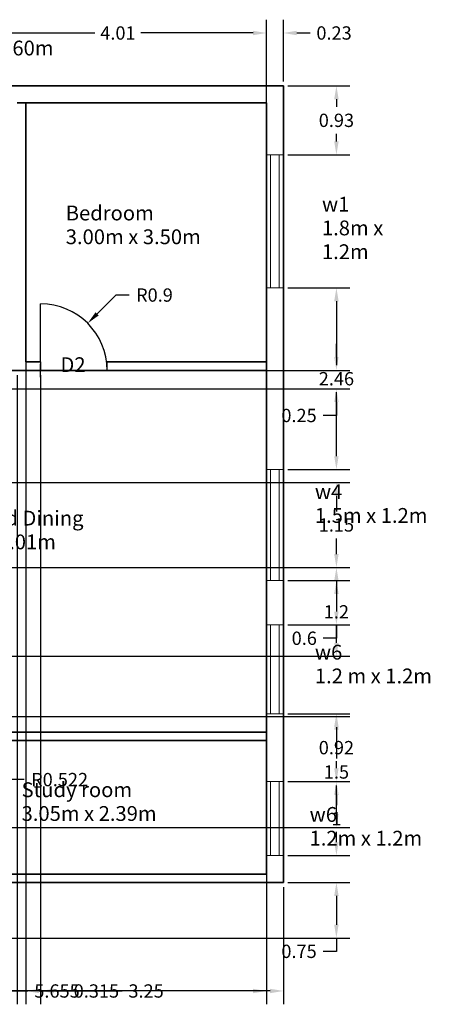
# Model space of a CAD drawing. Units: metres. Extents: x 1585.4 to 1599.4, y 2063.3 to 2076.9.
# Tile 3 of 3: x 1593.9 to 1599.4, y 2063.3 to 2076.6. Entities that reach past the tile are written whole.
import ezdxf

# ---------------------------------------------------------------- set-up
doc = ezdxf.new("R2010")
doc.units = ezdxf.units.M
for name, color, linetype, lineweight in [('A-ANNO-DIMS', 2, 'Continuous', 18), ('A-ANNO-TEXT', 7, 'Continuous', 18), ('A-AREA-IDEN', 7, 'Continuous', 18), ('A-DOOR', 3, 'Continuous', 25), ('A-GLAZ', 4, 'Continuous', 18), ('A-WALL', 7, 'Continuous', 35)]:
    doc.layers.add(name, color=color, linetype=linetype, lineweight=lineweight)
doc.styles.get("Standard").update_dxf_attribs({"font": 'arial.ttf'})
doc.dimstyles.get("Standard").update_dxf_attribs({"dimtxt": 0.18, "dimasz": 0.18, "dimexe": 0.18, "dimexo": 0.0625, "dimgap": 0.09, "dimtad": 0, "dimtih": 1, "dimtoh": 1, "dimdec": 4, "dimzin": 0, "dimdsep": 46, "dimtxsty": 'Standard', "dimcen": 0.09, "dimadec": 0, "dimazin": 0, "dimtfac": 1, "dimtdec": 4, "dimtofl": 0, "dimtmove": 0, "dimatfit": 3, "dimfxl": 1, "dimtolj": 1, "dimtzin": 0, "dimarcsym": 0})

# ---------------------------------------------------------------- blocks, each defined once
blk = doc.blocks.new('WIN-FRAME-1800')
for p, q in [((0, 0), (0, 0.23)), ((0, 0.23), (1.8, 0.23)), ((1.8, 0.23), (1.8, 0))]:
    blk.add_line(p, q)
blk = doc.blocks.new('WIN-FRAME-1500')
for p, q in [((0, 0), (0, 0.23)), ((0, 0.23), (1.5, 0.23)), ((1.5, 0.23), (1.5, 0))]:
    blk.add_line(p, q)
blk = doc.blocks.new('WIN-FRAME-1000')
for p, q in [((0, 0), (0, 1)), ((0, 1), (0.23, 1)), ((0.23, 0), (0, 0))]:
    blk.add_line(p, q)
blk = doc.blocks.new('WIN-FRAME-1200')
for p, q in [((0, 0), (0, 1.2)), ((0, 1.2), (0.23, 1.2)), ((0.23, 0), (0, 0))]:
    blk.add_line(p, q)
blk = doc.blocks.new('*D6')
at = {"layer": 'A-ANNO-DIMS', "color": 0, "lineweight": -2, "transparency": 16777216}
for p, q in [((1586.931, 2064.876), (1586.931, 2063.293)), ((1597.431, 2064.876), (1597.431, 2063.293)), ((1587.111, 2063.473), (1591.865, 2063.473)), ((1597.251, 2063.473), (1592.497, 2063.473))]:
    blk.add_line(p, q, dxfattribs=at)
at = {"layer": 'A-ANNO-DIMS', "color": 0, "transparency": 16777216}
for points in [[(1587.111, 2063.503), (1587.111, 2063.443), (1586.931, 2063.473)], [(1597.251, 2063.503), (1597.251, 2063.443), (1597.431, 2063.473)]]:
    blk.add_solid(points, dxfattribs=at)
at = {"layer": 'Defpoints', "color": 0, "transparency": 16777216}
for p in [(1586.931, 2064.939), (1597.431, 2064.939), (1597.431, 2063.473)]:
    blk.add_point(p, dxfattribs=at)
at = {"layer": 'A-ANNO-DIMS', "color": 0, "transparency": 16777216, "insert": (1592.181, 2063.473), "char_height": 0.18, "attachment_point": 5}
blk.add_mtext('\\A1;10.5', dxfattribs=at)
blk = doc.blocks.new('*D9')
at = {"layer": 'A-ANNO-DIMS', "color": 0, "lineweight": -2, "transparency": 16777216}
for p, q in [((1597.201, 2075.541), (1597.201, 2076.605)), ((1597.431, 2075.771), (1597.431, 2076.605)), ((1597.021, 2076.425), (1596.841, 2076.425)), ((1597.611, 2076.425), (1597.791, 2076.425))]:
    blk.add_line(p, q, dxfattribs=at)
at = {"layer": 'A-ANNO-DIMS', "color": 0, "transparency": 16777216}
for points in [[(1597.021, 2076.455), (1597.021, 2076.395), (1597.201, 2076.425)], [(1597.611, 2076.455), (1597.611, 2076.395), (1597.431, 2076.425)]]:
    blk.add_solid(points, dxfattribs=at)
at = {"layer": 'Defpoints', "color": 0, "transparency": 16777216}
for p in [(1597.431, 2076.425), (1597.431, 2075.709), (1597.201, 2075.479)]:
    blk.add_point(p, dxfattribs=at)
at = {"layer": 'A-ANNO-DIMS', "color": 0, "transparency": 16777216, "insert": (1598.115, 2076.425), "char_height": 0.18, "attachment_point": 5}
blk.add_mtext('\\A1;0.23', dxfattribs=at)
blk = doc.blocks.new('*D10')
at = {"layer": 'A-ANNO-DIMS', "color": 0, "lineweight": -2, "transparency": 16777216}
for p, q in [((1597.493, 2064.939), (1598.327, 2064.939)), ((1598.147, 2064.759), (1598.147, 2064.369)), ((1593.112, 2064.189), (1598.327, 2064.189)), ((1598.147, 2064.189), (1598.147, 2064.009)), ((1598.147, 2064.009), (1597.967, 2064.009))]:
    blk.add_line(p, q, dxfattribs=at)
at = {"layer": 'A-ANNO-DIMS', "color": 0, "transparency": 16777216}
for points in [[(1598.117, 2064.759), (1598.177, 2064.759), (1598.147, 2064.939)], [(1598.117, 2064.369), (1598.177, 2064.369), (1598.147, 2064.189)]]:
    blk.add_solid(points, dxfattribs=at)
at = {"layer": 'Defpoints', "color": 0, "transparency": 16777216}
for p in [(1597.431, 2064.939), (1593.05, 2064.189), (1598.147, 2064.189)]:
    blk.add_point(p, dxfattribs=at)
at = {"layer": 'A-ANNO-DIMS', "color": 0, "transparency": 16777216, "insert": (1597.642, 2064.009), "char_height": 0.18, "attachment_point": 5}
blk.add_mtext('\\A1;0.75', dxfattribs=at)
blk = doc.blocks.new('*D14')
at = {"layer": 'A-ANNO-DIMS', "color": 0, "lineweight": -2, "transparency": 16777216}
for p, q in [((1597.493, 2075.709), (1598.327, 2075.709)), ((1598.147, 2075.529), (1598.147, 2075.426)), ((1598.147, 2074.959), (1598.147, 2075.062)), ((1597.493, 2074.779), (1598.327, 2074.779))]:
    blk.add_line(p, q, dxfattribs=at)
at = {"layer": 'A-ANNO-DIMS', "color": 0, "transparency": 16777216}
for points in [[(1598.117, 2075.529), (1598.177, 2075.529), (1598.147, 2075.709)], [(1598.117, 2074.959), (1598.177, 2074.959), (1598.147, 2074.779)]]:
    blk.add_solid(points, dxfattribs=at)
at = {"layer": 'Defpoints', "color": 0, "transparency": 16777216}
for p in [(1597.431, 2075.709), (1597.431, 2074.779), (1598.147, 2074.779)]:
    blk.add_point(p, dxfattribs=at)
at = {"layer": 'A-ANNO-DIMS', "color": 0, "transparency": 16777216, "insert": (1598.147, 2075.244), "char_height": 0.18, "attachment_point": 5}
blk.add_mtext('\\A1;0.93', dxfattribs=at)
blk = doc.blocks.new('*D15')
at = {"layer": 'A-ANNO-DIMS', "color": 0, "lineweight": -2, "transparency": 16777216}
for p, q in [((1597.493, 2072.979), (1598.327, 2072.979)), ((1598.147, 2072.799), (1598.147, 2071.932)), ((1598.147, 2070.702), (1598.147, 2071.569)), ((1597.493, 2070.522), (1598.327, 2070.522))]:
    blk.add_line(p, q, dxfattribs=at)
at = {"layer": 'A-ANNO-DIMS', "color": 0, "transparency": 16777216}
for points in [[(1598.117, 2072.799), (1598.177, 2072.799), (1598.147, 2072.979)], [(1598.117, 2070.702), (1598.177, 2070.702), (1598.147, 2070.522)]]:
    blk.add_solid(points, dxfattribs=at)
at = {"layer": 'Defpoints', "color": 0, "transparency": 16777216}
for p in [(1597.431, 2072.979), (1597.431, 2070.522), (1598.147, 2070.522)]:
    blk.add_point(p, dxfattribs=at)
at = {"layer": 'A-ANNO-DIMS', "color": 0, "transparency": 16777216, "insert": (1598.147, 2071.751), "char_height": 0.18, "attachment_point": 5}
blk.add_mtext('\\A1;2.46', dxfattribs=at)
blk = doc.blocks.new('*D16')
at = {"layer": 'A-ANNO-DIMS', "color": 0, "lineweight": -2, "transparency": 16777216}
for p, q in [((1597.493, 2069.022), (1598.327, 2069.022)), ((1598.147, 2068.842), (1598.147, 2068.602)), ((1597.493, 2068.422), (1598.327, 2068.422)), ((1598.147, 2068.422), (1598.147, 2068.242)), ((1598.147, 2068.242), (1597.967, 2068.242))]:
    blk.add_line(p, q, dxfattribs=at)
at = {"layer": 'A-ANNO-DIMS', "color": 0, "transparency": 16777216}
for points in [[(1598.117, 2068.842), (1598.177, 2068.842), (1598.147, 2069.022)], [(1598.117, 2068.602), (1598.177, 2068.602), (1598.147, 2068.422)]]:
    blk.add_solid(points, dxfattribs=at)
at = {"layer": 'Defpoints', "color": 0, "transparency": 16777216}
for p in [(1597.431, 2069.022), (1597.431, 2068.422), (1598.147, 2068.422)]:
    blk.add_point(p, dxfattribs=at)
at = {"layer": 'A-ANNO-DIMS', "color": 0, "transparency": 16777216, "insert": (1597.713, 2068.242), "char_height": 0.18, "attachment_point": 5}
blk.add_mtext('\\A1;0.6', dxfattribs=at)
blk = doc.blocks.new('*D17')
at = {"layer": 'A-ANNO-DIMS', "color": 0, "lineweight": -2, "transparency": 16777216}
for p, q in [((1597.493, 2067.222), (1598.327, 2067.222)), ((1598.147, 2067.042), (1598.147, 2066.945)), ((1598.147, 2066.484), (1598.147, 2066.581)), ((1597.493, 2066.304), (1598.327, 2066.304))]:
    blk.add_line(p, q, dxfattribs=at)
at = {"layer": 'A-ANNO-DIMS', "color": 0, "transparency": 16777216}
for points in [[(1598.117, 2067.042), (1598.177, 2067.042), (1598.147, 2067.222)], [(1598.117, 2066.484), (1598.177, 2066.484), (1598.147, 2066.304)]]:
    blk.add_solid(points, dxfattribs=at)
at = {"layer": 'Defpoints', "color": 0, "transparency": 16777216}
for p in [(1597.431, 2067.222), (1597.431, 2066.304), (1598.147, 2066.304)]:
    blk.add_point(p, dxfattribs=at)
at = {"layer": 'A-ANNO-DIMS', "color": 0, "transparency": 16777216, "insert": (1598.147, 2066.763), "char_height": 0.18, "attachment_point": 5}
blk.add_mtext('\\A1;0.92', dxfattribs=at)
blk = doc.blocks.new('*D18')
at = {"layer": 'A-ANNO-DIMS', "color": 0, "lineweight": -2, "transparency": 16777216}
for p, q in [((1597.493, 2066.304), (1598.327, 2066.304)), ((1598.147, 2066.124), (1598.147, 2065.984)), ((1598.147, 2065.484), (1598.147, 2065.623)), ((1597.493, 2065.304), (1598.327, 2065.304))]:
    blk.add_line(p, q, dxfattribs=at)
at = {"layer": 'A-ANNO-DIMS', "color": 0, "transparency": 16777216}
for points in [[(1598.117, 2066.124), (1598.177, 2066.124), (1598.147, 2066.304)], [(1598.117, 2065.484), (1598.177, 2065.484), (1598.147, 2065.304)]]:
    blk.add_solid(points, dxfattribs=at)
at = {"layer": 'Defpoints', "color": 0, "transparency": 16777216}
for p in [(1597.431, 2066.304), (1597.431, 2065.304), (1598.147, 2065.304)]:
    blk.add_point(p, dxfattribs=at)
at = {"layer": 'A-ANNO-DIMS', "color": 0, "transparency": 16777216, "insert": (1598.147, 2065.804), "char_height": 0.18, "attachment_point": 5}
blk.add_mtext('\\A1;1', dxfattribs=at)
blk = doc.blocks.new('*D19')
at = {"layer": 'A-ANNO-DIMS', "color": 0, "lineweight": -2, "transparency": 16777216}
for p, q in [((1587.223, 2070.349), (1598.327, 2070.349)), ((1598.147, 2070.169), (1598.147, 2069.956)), ((1598.147, 2069.379), (1598.147, 2069.592)), ((1587.223, 2069.199), (1598.327, 2069.199))]:
    blk.add_line(p, q, dxfattribs=at)
at = {"layer": 'A-ANNO-DIMS', "color": 0, "transparency": 16777216}
for points in [[(1598.117, 2070.169), (1598.177, 2070.169), (1598.147, 2070.349)], [(1598.117, 2069.379), (1598.177, 2069.379), (1598.147, 2069.199)]]:
    blk.add_solid(points, dxfattribs=at)
at = {"layer": 'Defpoints', "color": 0, "transparency": 16777216}
for p in [(1587.161, 2070.349), (1587.161, 2069.199), (1598.147, 2069.199)]:
    blk.add_point(p, dxfattribs=at)
at = {"layer": 'A-ANNO-DIMS', "color": 0, "transparency": 16777216, "insert": (1598.147, 2069.774), "char_height": 0.18, "attachment_point": 5}
blk.add_mtext('\\A1;1.15', dxfattribs=at)
blk = doc.blocks.new('*D20')
at = {"layer": 'A-ANNO-DIMS', "color": 0, "lineweight": -2, "transparency": 16777216}
for p, q in [((1587.223, 2069.199), (1598.327, 2069.199)), ((1598.147, 2069.019), (1598.147, 2068.779)), ((1598.147, 2068.179), (1598.147, 2068.418)), ((1587.223, 2067.999), (1598.327, 2067.999))]:
    blk.add_line(p, q, dxfattribs=at)
at = {"layer": 'A-ANNO-DIMS', "color": 0, "transparency": 16777216}
for points in [[(1598.117, 2069.019), (1598.177, 2069.019), (1598.147, 2069.199)], [(1598.117, 2068.179), (1598.177, 2068.179), (1598.147, 2067.999)]]:
    blk.add_solid(points, dxfattribs=at)
at = {"layer": 'Defpoints', "color": 0, "transparency": 16777216}
for p in [(1587.161, 2069.199), (1598.147, 2069.199), (1587.161, 2067.999)]:
    blk.add_point(p, dxfattribs=at)
at = {"layer": 'A-ANNO-DIMS', "color": 0, "transparency": 16777216, "insert": (1598.147, 2068.599), "char_height": 0.18, "attachment_point": 5}
blk.add_mtext('\\A1;1.2', dxfattribs=at)
blk = doc.blocks.new('*D21')
at = {"layer": 'A-ANNO-DIMS', "color": 0, "lineweight": -2, "transparency": 16777216}
for p, q in [((1598.147, 2072.044), (1598.147, 2072.224)), ((1587.223, 2071.864), (1598.327, 2071.864)), ((1587.223, 2071.614), (1598.327, 2071.614)), ((1598.147, 2071.434), (1598.147, 2071.254)), ((1598.147, 2071.254), (1597.967, 2071.254))]:
    blk.add_line(p, q, dxfattribs=at)
at = {"layer": 'A-ANNO-DIMS', "color": 0, "transparency": 16777216}
for points in [[(1598.117, 2072.044), (1598.177, 2072.044), (1598.147, 2071.864)], [(1598.117, 2071.434), (1598.177, 2071.434), (1598.147, 2071.614)]]:
    blk.add_solid(points, dxfattribs=at)
at = {"layer": 'Defpoints', "color": 0, "transparency": 16777216}
for p in [(1587.161, 2071.864), (1587.161, 2071.614), (1598.147, 2071.614)]:
    blk.add_point(p, dxfattribs=at)
at = {"layer": 'A-ANNO-DIMS', "color": 0, "transparency": 16777216, "insert": (1597.642, 2071.254), "char_height": 0.18, "attachment_point": 5}
blk.add_mtext('\\A1;0.25', dxfattribs=at)
blk = doc.blocks.new('*D24')
at = {"layer": 'A-ANNO-DIMS', "color": 0, "lineweight": -2, "transparency": 16777216}
for p, q in [((1593.951, 2075.416), (1593.951, 2063.293)), ((1597.201, 2075.416), (1597.201, 2063.293)), ((1594.131, 2063.473), (1595.251, 2063.473)), ((1597.021, 2063.473), (1595.9, 2063.473))]:
    blk.add_line(p, q, dxfattribs=at)
at = {"layer": 'A-ANNO-DIMS', "color": 0, "transparency": 16777216}
for points in [[(1594.131, 2063.503), (1594.131, 2063.443), (1593.951, 2063.473)], [(1597.021, 2063.503), (1597.021, 2063.443), (1597.201, 2063.473)]]:
    blk.add_solid(points, dxfattribs=at)
at = {"layer": 'Defpoints', "color": 0, "transparency": 16777216}
for p in [(1593.951, 2075.479), (1597.201, 2075.479), (1597.201, 2063.473)]:
    blk.add_point(p, dxfattribs=at)
at = {"layer": 'A-ANNO-DIMS', "color": 0, "transparency": 16777216, "insert": (1595.576, 2063.473), "char_height": 0.18, "attachment_point": 5}
blk.add_mtext('\\A1;3.25', dxfattribs=at)
blk = doc.blocks.new('*D25')
at = {"layer": 'A-ANNO-DIMS', "color": 0, "lineweight": -2, "transparency": 16777216}
for p, q in [((1597.138, 2066.857), (1586.035, 2066.857)), ((1586.215, 2066.677), (1586.215, 2066.137)), ((1586.215, 2065.234), (1586.215, 2065.774)), ((1597.138, 2065.054), (1586.035, 2065.054))]:
    blk.add_line(p, q, dxfattribs=at)
at = {"layer": 'A-ANNO-DIMS', "color": 0, "transparency": 16777216}
for points in [[(1586.185, 2066.677), (1586.245, 2066.677), (1586.215, 2066.857)], [(1586.185, 2065.234), (1586.245, 2065.234), (1586.215, 2065.054)]]:
    blk.add_solid(points, dxfattribs=at)
at = {"layer": 'Defpoints', "color": 0, "transparency": 16777216}
for p in [(1586.215, 2066.857), (1597.201, 2066.857), (1597.201, 2065.054)]:
    blk.add_point(p, dxfattribs=at)
at = {"layer": 'A-ANNO-DIMS', "color": 0, "transparency": 16777216, "insert": (1586.215, 2065.956), "char_height": 0.18, "attachment_point": 5}
blk.add_mtext('\\A1;1.80', dxfattribs=at)
blk = doc.blocks.new('*D26')
at = {"layer": 'A-ANNO-DIMS', "color": 0, "lineweight": -2, "transparency": 16777216}
for p, q in [((1593.191, 2065.116), (1593.191, 2076.605)), ((1597.201, 2065.116), (1597.201, 2076.605)), ((1593.371, 2076.425), (1594.886, 2076.425)), ((1597.021, 2076.425), (1595.506, 2076.425))]:
    blk.add_line(p, q, dxfattribs=at)
at = {"layer": 'A-ANNO-DIMS', "color": 0, "transparency": 16777216}
for points in [[(1593.371, 2076.455), (1593.371, 2076.395), (1593.191, 2076.425)], [(1597.021, 2076.455), (1597.021, 2076.395), (1597.201, 2076.425)]]:
    blk.add_solid(points, dxfattribs=at)
at = {"layer": 'Defpoints', "color": 0, "transparency": 16777216}
for p in [(1597.201, 2076.425), (1593.191, 2065.054), (1597.201, 2065.054)]:
    blk.add_point(p, dxfattribs=at)
at = {"layer": 'A-ANNO-DIMS', "color": 0, "transparency": 16777216, "insert": (1595.196, 2076.425), "char_height": 0.18, "attachment_point": 5}
blk.add_mtext('\\A1;4.01', dxfattribs=at)
blk = doc.blocks.new('*D29')
at = {"layer": 'A-ANNO-DIMS', "color": 0, "lineweight": -2, "transparency": 16777216}
for p, q in [((1590.216, 2067.184), (1598.327, 2067.184)), ((1598.147, 2067.004), (1598.147, 2066.616)), ((1598.147, 2065.864), (1598.147, 2066.252)), ((1590.216, 2065.684), (1598.327, 2065.684))]:
    blk.add_line(p, q, dxfattribs=at)
at = {"layer": 'A-ANNO-DIMS', "color": 0, "transparency": 16777216}
for points in [[(1598.117, 2067.004), (1598.177, 2067.004), (1598.147, 2067.184)], [(1598.117, 2065.864), (1598.177, 2065.864), (1598.147, 2065.684)]]:
    blk.add_solid(points, dxfattribs=at)
at = {"layer": 'Defpoints', "color": 0, "transparency": 16777216}
for p in [(1590.153, 2067.184), (1590.153, 2065.684), (1598.147, 2065.684)]:
    blk.add_point(p, dxfattribs=at)
at = {"layer": 'A-ANNO-DIMS', "color": 0, "transparency": 16777216, "insert": (1598.147, 2066.434), "char_height": 0.18, "attachment_point": 5}
blk.add_mtext('\\A1;1.5', dxfattribs=at)
blk = doc.blocks.new('*D31')
at = {"layer": 'A-ANNO-DIMS', "color": 0, "lineweight": -2, "transparency": 16777216}
for p, q in [((1593.836, 2071.801), (1593.836, 2063.293)), ((1594.151, 2071.801), (1594.151, 2063.293)), ((1593.656, 2063.473), (1593.476, 2063.473)), ((1594.331, 2063.473), (1594.511, 2063.473))]:
    blk.add_line(p, q, dxfattribs=at)
at = {"layer": 'A-ANNO-DIMS', "color": 0, "transparency": 16777216}
for points in [[(1593.656, 2063.503), (1593.656, 2063.443), (1593.836, 2063.473)], [(1594.331, 2063.503), (1594.331, 2063.443), (1594.151, 2063.473)]]:
    blk.add_solid(points, dxfattribs=at)
at = {"layer": 'Defpoints', "color": 0, "transparency": 16777216}
for p in [(1593.836, 2071.864), (1594.151, 2071.864), (1594.151, 2063.473)]:
    blk.add_point(p, dxfattribs=at)
at = {"layer": 'A-ANNO-DIMS', "color": 0, "transparency": 16777216, "insert": (1594.905, 2063.473), "char_height": 0.18, "attachment_point": 5}
blk.add_mtext('\\A1;0.315', dxfattribs=at)
blk = doc.blocks.new('*D36')
at = {"layer": 'A-ANNO-DIMS', "color": 0, "lineweight": -2, "transparency": 16777216}
for p, q in [((1597.201, 2070.46), (1597.201, 2063.293)), ((1591.546, 2070.401), (1591.546, 2063.293)), ((1591.726, 2063.473), (1593.979, 2063.473)), ((1597.021, 2063.473), (1594.768, 2063.473))]:
    blk.add_line(p, q, dxfattribs=at)
at = {"layer": 'A-ANNO-DIMS', "color": 0, "transparency": 16777216}
for points in [[(1591.726, 2063.503), (1591.726, 2063.443), (1591.546, 2063.473)], [(1597.021, 2063.503), (1597.021, 2063.443), (1597.201, 2063.473)]]:
    blk.add_solid(points, dxfattribs=at)
at = {"layer": 'Defpoints', "color": 0, "transparency": 16777216}
for p in [(1591.546, 2070.464), (1597.201, 2070.522), (1597.201, 2063.473)]:
    blk.add_point(p, dxfattribs=at)
at = {"layer": 'A-ANNO-DIMS', "color": 0, "transparency": 16777216, "insert": (1594.373, 2063.473), "char_height": 0.18, "attachment_point": 5}
blk.add_mtext('\\A1;5.655', dxfattribs=at)
blk = doc.blocks.new('*D37')
at = {"layer": 'A-ANNO-DIMS', "color": 0, "lineweight": -2, "transparency": 16777216}
for p, q in [((1597.138, 2071.864), (1586.035, 2071.864)), ((1586.215, 2071.684), (1586.215, 2069.6)), ((1586.215, 2067.152), (1586.215, 2069.236)), ((1597.138, 2066.972), (1586.035, 2066.972))]:
    blk.add_line(p, q, dxfattribs=at)
at = {"layer": 'A-ANNO-DIMS', "color": 0, "transparency": 16777216}
for points in [[(1586.185, 2071.684), (1586.245, 2071.684), (1586.215, 2071.864)], [(1586.185, 2067.152), (1586.245, 2067.152), (1586.215, 2066.972)]]:
    blk.add_solid(points, dxfattribs=at)
at = {"layer": 'Defpoints', "color": 0, "transparency": 16777216}
for p in [(1586.215, 2071.864), (1597.201, 2071.864), (1597.201, 2066.972)]:
    blk.add_point(p, dxfattribs=at)
at = {"layer": 'A-ANNO-DIMS', "color": 0, "transparency": 16777216, "insert": (1586.215, 2069.418), "char_height": 0.18, "attachment_point": 5}
blk.add_mtext('\\A1;4.892', dxfattribs=at)
blk = doc.blocks.new('*D39')
at = {"layer": 'A-ANNO-DIMS', "color": 0, "lineweight": -2, "transparency": 16777216}
for p, q in [((1595.169, 2072.882), (1594.915, 2072.628)), ((1595.349, 2072.882), (1595.169, 2072.882)), ((1594.151, 2071.774), (1594.151, 2071.954)), ((1594.061, 2071.864), (1594.241, 2071.864))]:
    blk.add_line(p, q, dxfattribs=at)
at = {"layer": 'A-ANNO-DIMS', "color": 0, "transparency": 16777216}
blk.add_solid([(1594.893, 2072.649), (1594.936, 2072.606), (1594.787, 2072.5)], dxfattribs=at)
at = {"layer": 'Defpoints', "color": 0, "transparency": 16777216}
for p in [(1594.787, 2072.5), (1594.151, 2071.864)]:
    blk.add_point(p, dxfattribs=at)
at = {"layer": 'A-ANNO-DIMS', "color": 0, "transparency": 16777216, "insert": (1595.689, 2072.882), "char_height": 0.18, "attachment_point": 5}
blk.add_mtext('\\A1;R0.9', dxfattribs=at)
blk = doc.blocks.new('*D43')
at = {"layer": 'A-ANNO-DIMS', "color": 0, "lineweight": -2, "transparency": 16777216}
for p, q in [((1592.951, 2066.857), (1593.131, 2066.857)), ((1593.041, 2066.767), (1593.041, 2066.947)), ((1593.749, 2066.331), (1593.604, 2066.439)), ((1593.929, 2066.331), (1593.749, 2066.331))]:
    blk.add_line(p, q, dxfattribs=at)
at = {"layer": 'A-ANNO-DIMS', "color": 0, "transparency": 16777216}
blk.add_solid([(1593.622, 2066.463), (1593.587, 2066.415), (1593.46, 2066.546)], dxfattribs=at)
at = {"layer": 'Defpoints', "color": 0, "transparency": 16777216}
for p in [(1593.041, 2066.857), (1593.46, 2066.546)]:
    blk.add_point(p, dxfattribs=at)
at = {"layer": 'A-ANNO-DIMS', "color": 0, "transparency": 16777216, "insert": (1594.408, 2066.331), "char_height": 0.18, "attachment_point": 5}
blk.add_mtext('\\A1;R0.522', dxfattribs=at)

msp = doc.modelspace()

# ---------------------------------------------------------------- linework, layer by layer
at = {"layer": 'A-DOOR'}
for p, q in [((1594.1508, 2071.9788), (1594.1508, 2072.7638)), ((1594.1508, 2071.9788), (1594.1508, 2071.8638)), ((1595.0508, 2071.8638), (1595.0508, 2071.9788))]:
    msp.add_line(p, q, dxfattribs=at)
msp.add_arc((1594.1508, 2071.8638), 0.9, 0, 90, dxfattribs=at)
at = {"layer": 'A-GLAZ'}
for p, q in [((1597.2008, 2072.9788), (1597.2008, 2074.7788)), ((1597.2558, 2072.9788), (1597.2558, 2074.7788)), ((1597.3758, 2072.9788), (1597.3758, 2074.7788)), ((1597.2558, 2069.0223), (1597.2558, 2070.5223)), ((1597.3758, 2069.0223), (1597.3758, 2070.5223)), ((1597.2558, 2067.2223), (1597.2558, 2068.4223)), ((1597.3758, 2067.2223), (1597.3758, 2068.4223)), ((1597.2008, 2065.3038), (1597.2008, 2066.3038)), ((1597.2558, 2065.3038), (1597.2558, 2066.3038)), ((1597.3758, 2065.3038), (1597.3758, 2066.3038))]:
    msp.add_line(p, q, dxfattribs=at)
at = {"layer": 'A-WALL'}
for p, q in [((1597.4308, 2075.7088), (1597.2008, 2075.7088)), ((1593.9508, 2075.4788), (1593.8358, 2075.4788)), ((1597.2008, 2075.4788), (1593.9508, 2075.4788)), ((1593.9508, 2075.4788), (1593.9508, 2071.9788)), ((1597.2008, 2071.9788), (1597.2008, 2075.4788)), ((1597.2008, 2071.9788), (1597.2008, 2072.9788)), ((1593.9508, 2071.9788), (1594.1508, 2071.9788)), ((1593.9508, 2071.9788), (1594.1508, 2071.9788)), ((1595.0508, 2071.9788), (1597.2008, 2071.9788)), ((1597.2008, 2071.9788), (1597.2008, 2071.9788)), ((1593.8358, 2071.8638), (1594.1508, 2071.8638)), ((1595.0508, 2071.8638), (1597.2008, 2071.8638)), ((1597.2008, 2071.8638), (1597.2008, 2066.9723)), ((1597.2008, 2068.4223), (1597.2008, 2069.0223)), ((1597.2008, 2068.4223), (1597.2008, 2068.4223)), ((1597.2008, 2066.9723), (1597.2008, 2067.3288)), ((1597.2008, 2066.9723), (1597.2008, 2067.2223)), ((1597.2008, 2066.9723), (1593.0408, 2066.9723)), ((1593.1908, 2066.8573), (1597.2008, 2066.8573)), ((1597.2008, 2065.0538), (1597.2008, 2066.8573)), ((1597.2008, 2066.8573), (1597.2008, 2065.0538)), ((1597.2008, 2065.0538), (1597.2008, 2065.3038)), ((1597.2008, 2065.0538), (1593.1908, 2065.0538)), ((1593.0458, 2064.9388), (1597.2008, 2064.9388)), ((1597.2008, 2064.9388), (1597.4308, 2064.9388))]:
    msp.add_line(p, q, dxfattribs=at)
msp.add_lwpolyline([(1597.4308, 2064.9388), (1597.4308, 2075.7088), (1586.9308, 2075.7088), (1586.9308, 2064.9388)], dxfattribs=at)

# ---------------------------------------------------------------- block references
at = {"layer": 'A-GLAZ'}
for name, p, rotation in [('WIN-FRAME-1800', (1597.2008, 2074.7788), 269.9999999999952), ('WIN-FRAME-1500', (1597.2008, 2070.5223), 270), ('WIN-FRAME-1200', (1597.4308, 2068.4223), 180), ('WIN-FRAME-1000', (1597.4308, 2066.3038), 180)]:
    msp.add_blockref(name, p, dxfattribs=dict(at, rotation=rotation))

# ---------------------------------------------------------------- texts
at = {"layer": 'A-ANNO-TEXT'}
for s, p in [('0.9m x 0.60m', (1592.6536, 2076.1214)), ('w1', (1597.9517, 2074.0105)), ('1.8m x', (1597.9517, 2073.6892)), ('1.2m', (1597.9517, 2073.3679)), ('D2', (1594.4197, 2071.8405)), ('w4', (1597.8563, 2070.1236)), ('1.5m x 1.2m', (1597.8563, 2069.8023)), ('w6', (1597.8563, 2067.9537)), ('1.2 m x 1.2m', (1597.8563, 2067.6324)), ('w6', (1597.7847, 2065.7599)), ('1.2m x 1.2m', (1597.7847, 2065.4386))]:
    msp.add_text(s, height=0.2, dxfattribs=at).set_placement(p)
at = {"layer": 'A-AREA-IDEN'}
for s, p in [('Bedroom', (1594.4913, 2073.8912)), ('3.00m x 3.50m', (1594.4913, 2073.57)), ('Living and Dining', (1592.5343, 2069.7659)), ('4.57m x 7.01m', (1592.5343, 2069.4447)), ('Study room', (1593.8946, 2066.0937)), ('3.05m x 2.39m', (1593.8946, 2065.7724))]:
    msp.add_text(s, height=0.2, dxfattribs=at).set_placement(p)

# ---------------------------------------------------------------- dimensions: what is measured, and where the dimension line sits
at = {"layer": 'A-ANNO-DIMS'}
for base, p1, p2, override, picture, middle in [((1597.2008, 2076.4248), (1593.1908, 2065.0538), (1597.2008, 2065.0538), {"dimdec": 2, "dimlfac": 1, "dimrnd": 0, "dimzin": 0, "dimdsep": 46, "dimlunit": 2}, '*D26', (1595.1958, 2076.4248)), ((1597.4308, 2076.4248), (1597.2008, 2075.4788), (1597.4308, 2075.7088), {"dimdec": 2, "dimlfac": 1, "dimrnd": 0, "dimzin": 0, "dimdsep": 46, "dimlunit": 2}, '*D9', (1598.1146, 2076.4248)), ((1597.2008, 2063.4728), (1593.9508, 2075.4788), (1597.2008, 2075.4788), {"dimdec": 2, "dimlfac": 1, "dimrnd": 0, "dimzin": 0, "dimdsep": 46, "dimlunit": 2}, '*D24', (1595.5758, 2063.4728)), ((1594.1508, 2063.4728), (1593.8358, 2071.8638), (1594.1508, 2071.8638), {"dimdec": 3, "dimlfac": 1, "dimrnd": 0, "dimzin": 0, "dimdsep": 46, "dimlunit": 2}, '*D31', (1594.9052, 2063.4728)), ((1597.2008, 2063.4728), (1591.5458, 2070.4638), (1597.2008, 2070.5223), {"dimdec": 3, "dimlfac": 1, "dimrnd": 0, "dimzin": 0, "dimdsep": 46, "dimlunit": 2}, '*D36', (1594.3733, 2063.4728)), ((1597.4308, 2063.4728), (1586.9308, 2064.9388), (1597.4308, 2064.9388), {"dimdec": 1, "dimlfac": 1, "dimrnd": 0, "dimzin": 0, "dimdsep": 46, "dimlunit": 2}, '*D6', (1592.1808, 2063.4728))]:
    dim = msp.add_linear_dim(base=base, p1=p1, p2=p2, dimstyle='Standard', override=override, dxfattribs=at)
    dim.commit()
    dim.dimension.update_dxf_attribs({"geometry": picture, "text_midpoint": middle})
for base, p1, p2, override, picture, middle in [((1598.1468, 2074.7788), (1597.4308, 2075.7088), (1597.4308, 2074.7788), {"dimdec": 2, "dimlfac": 1, "dimrnd": 0, "dimzin": 0, "dimdsep": 46, "dimlunit": 2}, '*D14', (1598.1468, 2075.2438)), ((1598.1468, 2070.5223), (1597.4308, 2072.9788), (1597.4308, 2070.5223), {"dimdec": 2, "dimlfac": 1, "dimrnd": 0, "dimzin": 0, "dimdsep": 46, "dimlunit": 2}, '*D15', (1598.1468, 2071.7506)), ((1598.1468, 2071.6138), (1587.1608, 2071.8638), (1587.1608, 2071.6138), {"dimdec": 2, "dimlfac": 1, "dimrnd": 0, "dimzin": 0, "dimdsep": 46, "dimlunit": 2}, '*D21', (1597.6424, 2071.2538)), ((1586.21482, 2071.86384), (1597.20082, 2066.97232), (1597.20082, 2071.86384), {"dimdec": 3, "dimlfac": 1, "dimrnd": 0, "dimzin": 0, "dimdsep": 46, "dimlunit": 2}, '*D37', (1586.21482, 2069.41808)), ((1598.1468, 2069.1988), (1587.1608, 2070.3488), (1587.1608, 2069.1988), {"dimdec": 2, "dimlfac": 1, "dimrnd": 0, "dimzin": 0, "dimdsep": 46, "dimlunit": 2}, '*D19', (1598.1468, 2069.7738)), ((1598.1468, 2069.1988), (1587.1608, 2067.9988), (1587.1608, 2069.1988), {"dimdec": 1, "dimlfac": 1, "dimrnd": 0, "dimzin": 0, "dimdsep": 46, "dimlunit": 2}, '*D20', (1598.1468, 2068.5988)), ((1598.1468, 2068.4223), (1597.4308, 2069.0223), (1597.4308, 2068.4223), {"dimdec": 1, "dimlfac": 1, "dimrnd": 0, "dimzin": 0, "dimdsep": 46, "dimlunit": 2}, '*D16', (1597.713, 2068.2423)), ((1598.1468, 2066.3038), (1597.4308, 2067.2223), (1597.4308, 2066.3038), {"dimdec": 2, "dimlfac": 1, "dimrnd": 0, "dimzin": 0, "dimdsep": 46, "dimlunit": 2}, '*D17', (1598.1468, 2066.7631)), ((1598.1468, 2065.6838), (1590.1533, 2067.1838), (1590.1533, 2065.6838), {"dimdec": 1, "dimlfac": 1, "dimrnd": 0, "dimzin": 0, "dimdsep": 46, "dimlunit": 2}, '*D29', (1598.1468, 2066.4338)), ((1586.2148, 2066.8573), (1597.2008, 2065.0538), (1597.2008, 2066.8573), {"dimdec": 2, "dimlfac": 1, "dimrnd": 0, "dimzin": 0, "dimdsep": 46, "dimlunit": 2}, '*D25', (1586.2148, 2065.9556)), ((1598.1468, 2065.3038), (1597.4308, 2066.3038), (1597.4308, 2065.3038), {"dimdec": 0, "dimlfac": 1, "dimrnd": 0, "dimzin": 0, "dimdsep": 46, "dimlunit": 2}, '*D18', (1598.1468, 2065.8038)), ((1598.1468, 2064.1888), (1597.4308, 2064.9388), (1593.0499, 2064.1888), {"dimdec": 2, "dimlfac": 1, "dimrnd": 0, "dimzin": 0, "dimdsep": 46, "dimlunit": 2}, '*D10', (1597.6424, 2064.0088))]:
    dim = msp.add_linear_dim(base=base, p1=p1, p2=p2, angle=90, dimstyle='Standard', override=override, dxfattribs=at)
    dim.commit()
    dim.dimension.update_dxf_attribs({"geometry": picture, "text_midpoint": middle})
dim = msp.add_radius_dim(center=(1594.1508, 2071.8638), mpoint=(1594.7872, 2072.5002), dimstyle='Standard', override={"dimdec": 1, "dimlfac": 1, "dimrnd": 0, "dimzin": 0, "dimdsep": 46, "dimlunit": 2}, dxfattribs=at)
dim.commit()
dim.dimension.update_dxf_attribs({"geometry": '*D39', "text_midpoint": (1595.6892, 2072.8821), "dimtype": 164})
dim = msp.add_radius_dim(center=(1593.0408, 2066.8573), mpoint=(1593.4599, 2066.5461), dimstyle='Standard', override={"dimdec": 3, "dimlfac": 1, "dimrnd": 0, "dimzin": 0, "dimdsep": 46, "dimlunit": 2}, dxfattribs=at)
dim.commit()
dim.dimension.update_dxf_attribs({"geometry": '*D43', "text_midpoint": (1594.4078, 2066.3314)})

doc.saveas('drawing.dxf')
